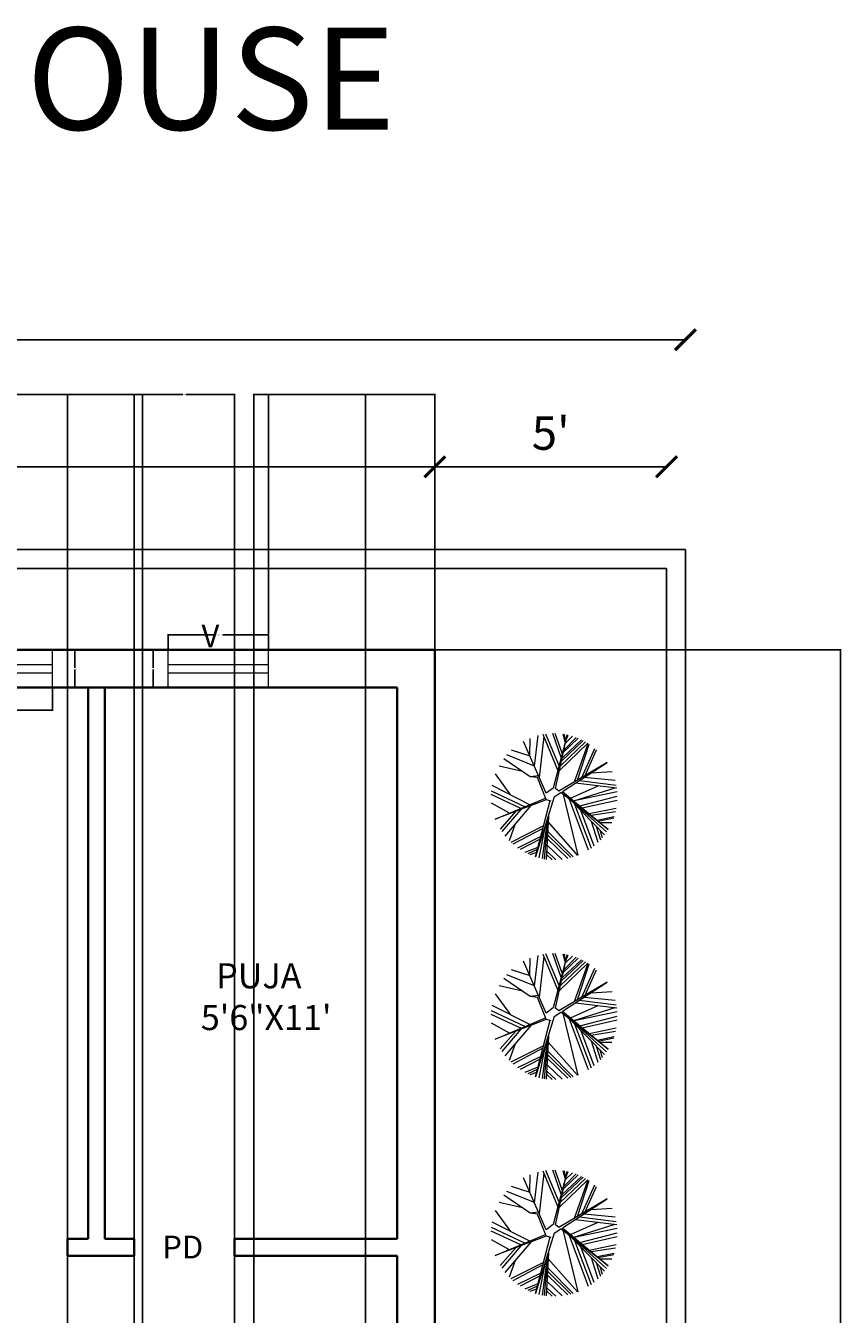
# Model space of a CAD drawing. Units: inches. Extents: x 503 to 1084, y -605 to 132.
# Tile 14 of 14: x 888 to 1084, y -177 to 132. Entities that reach past the tile are written whole.
import ezdxf

# ---------------------------------------------------------------- set-up
doc = ezdxf.new("R2010")
doc.units = ezdxf.units.IN
doc.header["$MEASUREMENT"] = 0
for name, color, linetype, lineweight in [('A-ANNO-DIMS', 7, 'Continuous', 18), ('A-ANNO-TEXT', 7, 'Continuous', 18), ('A-AREA-IDEN', 8, 'Continuous', 18), ('C-PROP', 1, 'Continuous', 25), ('wall', 1, 'Continuous', 35), ('wind', 5, 'Continuous', 18)]:
    doc.layers.add(name, color=color, linetype=linetype, lineweight=lineweight)
doc.layers.add('GRASS', color=90, linetype='Continuous', lineweight=13, transparency=0.7)
doc.styles.get("Standard").update_dxf_attribs({"font": 'arial.ttf'})
doc.dimstyles.get("Standard").update_dxf_attribs({"dimtxt": 0.18, "dimasz": 0.18, "dimexe": 0.18, "dimexo": 0.0625, "dimgap": 0.09, "dimtad": 0, "dimtih": 1, "dimtoh": 1, "dimdec": 1, "dimzin": 0, "dimdsep": 46, "dimlunit": 4, "dimtxsty": 'Standard', "dimcen": 0.09, "dimadec": 0, "dimazin": 0, "dimtfac": 1, "dimtdec": 1, "dimtofl": 0, "dimtmove": 0, "dimatfit": 3, "dimfxl": 1, "dimtolj": 1, "dimtzin": 0, "dimarcsym": 0})

# ---------------------------------------------------------------- blocks, each defined once
blk = doc.blocks.new('A$C4FA53466')
at = {"color": 0}
for p, q in [((0.717, 0.864), (0.422, 1.538)), ((0.501, 1.356), (0.505, 1.578)), ((0.563, 1.216), (0.612, 1.614)), ((0.627, 1.07), (0.687, 1.601)), ((0.867, 1.166), (0.675, 1.628)), ((0.882, 1.223), (0.709, 1.633)), ((0.91, 1.328), (0.802, 1.64)), ((0.988, 1.623), (0.804, 0.931)), ((0.925, 1.384), (0.834, 1.64)), ((0.836, 0.927), (0.988, 1.623)), ((0.887, 1.159), (1.256, 1.515)), ((0.901, 1.223), (1.228, 1.532)), ((0.914, 1.283), (1.197, 1.549)), ((0.922, 1.323), (1.176, 1.559)), ((0.964, 1.534), (0.938, 1.632)), ((0.938, 1.393), (1.132, 1.579)), ((0.945, 1.425), (1.104, 1.59)), ((0.967, 1.545), (0.952, 1.63)), ((0.965, 1.517), (1.059, 1.605)), ((0.974, 1.559), (1.002, 1.62)), ((1.085, 1.015), (1.262, 1.512)), ((0.562, 1.217), (0.205, 1.363)), ((0.505, 1.347), (0.266, 1.426)), ((1.121, 1.036), (1.274, 1.503)), ((1.18, 1.071), (1.349, 1.447)), ((1.222, 1.096), (1.37, 1.428)), ((0.406, 1.148), (0.102, 1.217)), ((0.506, 1.079), (0.165, 1.314)), ((1.509, 1.265), (0.879, 0.894)), ((0.926, 0.889), (1.509, 1.265)), ((0.255, 0.841), (0.055, 1.116)), ((0.614, 1.092), (0.506, 1.079)), ((0.604, 1.069), (0.506, 1.079)), ((0.715, 0.784), (0.604, 1.069)), ((1.148, 1.032), (1.626, 0.972)), ((1.211, 1.073), (1.612, 1.034)), ((1.3, 1.13), (1.573, 1.147)), ((0.384, 0.667), (0, 0.848)), ((0.436, 0.689), (0.003, 0.892)), ((0.501, 0.716), (0.012, 0.965)), ((0.804, 0.931), (0.717, 0.864)), ((0.82, 0.82), (0.904, 0.875)), ((0.879, 0.894), (0.836, 0.927)), ((1.521, 0.394), (0.904, 0.875)), ((0.926, 0.889), (1.521, 0.394)), ((0.938, 0.848), (1.126, 0.059)), ((1.03, 0.802), (1.392, 0.963)), ((1.073, 0.767), (1.614, 0.936)), ((1.081, 0.769), (1.638, 0.886)), ((1.097, 0.999), (1.632, 0.934)), ((0.237, 0.605), (0.004, 0.735)), ((0.053, 0.528), (0.708, 0.803)), ((0.716, 0.781), (0.053, 0.528)), ((0.516, 0.704), (0.179, 0.309)), ((0.82, 0.82), (0.575, 0.037)), ((0.575, 0.037), (0.769, 0.772)), ((0.715, 0.784), (0.775, 0.767)), ((1.016, 0.788), (1.263, 0.13)), ((1.04, 0.769), (1.475, 0.326)), ((1.06, 0.754), (1.5, 0.362)), ((1.083, 0.725), (1.298, 0.153)), ((1.153, 0.701), (1.64, 0.826)), ((1.185, 0.674), (1.639, 0.776)), ((1.273, 0.601), (1.627, 0.672)), ((0.321, 0.63), (0.115, 0.4)), ((0.387, 0.655), (0.137, 0.366)), ((0.732, 0.539), (0.664, 0.015)), ((0.737, 0.554), (0.691, 0.01)), ((0.744, 0.569), (0.717, 0.006)), ((1.161, 0.646), (1.335, 0.182)), ((1.298, 0.58), (1.618, 0.629)), ((1.301, 0.503), (1.386, 0.227)), ((1.376, 0.515), (1.599, 0.562)), ((1.392, 0.502), (1.593, 0.545)), ((0.313, 0.466), (0.232, 0.248)), ((0.682, 0.44), (0.255, 0.225)), ((0.673, 0.407), (0.281, 0.201)), ((0.701, 0.44), (0.621, 0.024)), ((0.735, 0.369), (1.067, 0.038)), ((0.74, 0.488), (1.121, 0.057)), ((1.365, 0.438), (1.42, 0.26)), ((1.412, 0.486), (1.569, 0.486)), ((1.413, 0.39), (1.444, 0.288)), ((0.645, 0.301), (0.342, 0.153)), ((0.636, 0.267), (0.375, 0.133)), ((0.726, 0.192), (0.924, 0.006)), ((0.73, 0.277), (0.998, 0.019)), ((0.733, 0.326), (1.037, 0.029)), ((0.608, 0.161), (0.439, 0.093)), ((0.6, 0.133), (0.475, 0.076)), ((0.59, 0.094), (0.501, 0.064)), ((0.72, 0.07), (0.793, 0)), ((0.722, 0.111), (0.842, 0))]:
    blk.add_line(p, q, dxfattribs=at)
blk = doc.blocks.new('_ArchTick')
at = {"color": 0, "linetype": 'ByBlock', "const_width": 0.15}
blk.add_lwpolyline([(-0.5, -0.5), (0.5, 0.5)], dxfattribs=at)
blk = doc.blocks.new('*D5')
at = {"layer": 'A-ANNO-DIMS', "color": 0, "lineweight": -3, "transparency": 16777216}
blk.add_line((590.09, 56.42), (1046.09, 56.42), dxfattribs=at)
at = {"layer": 'Defpoints', "color": 0, "transparency": 16777216}
for p in [(1046.09, 56.42), (590.09, 6.18), (1046.09, 6.18)]:
    blk.add_point(p, dxfattribs=at)
at = {"layer": 'A-ANNO-DIMS', "color": 0, "lineweight": -3, "transparency": 16777216, "xscale": 5, "yscale": 5, "zscale": 5, "rotation": 180}
blk.add_blockref('_ArchTick', (590.09, 56.42), dxfattribs=at)
at = {"layer": 'A-ANNO-DIMS', "color": 0, "lineweight": -3, "transparency": 16777216, "xscale": 5, "yscale": 5, "zscale": 5}
blk.add_blockref('_ArchTick', (1046.09, 56.42), dxfattribs=at)
at = {"layer": 'A-ANNO-DIMS', "color": 0, "transparency": 16777216, "insert": (818.09, 64.51), "char_height": 8, "attachment_point": 5}
blk.add_mtext("\\A1;38'", dxfattribs=at)
blk = doc.blocks.new('*D7')
at = {"layer": 'A-ANNO-DIMS', "color": 0, "lineweight": -3, "transparency": 16777216}
blk.add_line((650.09, 26.02), (986.09, 26.02), dxfattribs=at)
at = {"layer": 'Defpoints', "color": 0, "transparency": 16777216}
for p in [(986.09, 26.02), (650.09, -17.82), (986.09, -17.82)]:
    blk.add_point(p, dxfattribs=at)
at = {"layer": 'A-ANNO-DIMS', "color": 0, "lineweight": -3, "transparency": 16777216, "xscale": 5, "yscale": 5, "zscale": 5, "rotation": 180}
blk.add_blockref('_ArchTick', (650.09, 26.02), dxfattribs=at)
at = {"layer": 'A-ANNO-DIMS', "color": 0, "lineweight": -3, "transparency": 16777216, "xscale": 5, "yscale": 5, "zscale": 5}
blk.add_blockref('_ArchTick', (986.09, 26.02), dxfattribs=at)
at = {"layer": 'A-ANNO-DIMS', "color": 0, "transparency": 16777216, "insert": (818.09, 34.1), "char_height": 8, "attachment_point": 5}
blk.add_mtext("\\A1;28'", dxfattribs=at)
blk = doc.blocks.new('*D8')
at = {"layer": 'A-ANNO-DIMS', "color": 0, "lineweight": -3, "transparency": 16777216}
blk.add_line((986.09, 26.02), (1041.59, 26.02), dxfattribs=at)
at = {"layer": 'Defpoints', "color": 0, "transparency": 16777216}
for p in [(1041.59, 26.02), (986.09, -17.82), (1041.59, -17.14)]:
    blk.add_point(p, dxfattribs=at)
at = {"layer": 'A-ANNO-DIMS', "color": 0, "lineweight": -3, "transparency": 16777216, "xscale": 5, "yscale": 5, "zscale": 5, "rotation": 180}
blk.add_blockref('_ArchTick', (986.09, 26.02), dxfattribs=at)
at = {"layer": 'A-ANNO-DIMS', "color": 0, "lineweight": -3, "transparency": 16777216, "xscale": 5, "yscale": 5, "zscale": 5}
blk.add_blockref('_ArchTick', (1041.59, 26.02), dxfattribs=at)
at = {"layer": 'A-ANNO-DIMS', "color": 0, "transparency": 16777216, "insert": (1013.84, 34.09), "char_height": 8, "attachment_point": 5}
blk.add_mtext("\\A1;5'", dxfattribs=at)
blk = doc.blocks.new('WIN-36IN')
for p, q in [((0, 0), (0, 9)), ((36, 0), (36, 9)), ((0, 5.5), (36, 5.5)), ((0, 3.5), (36, 3.5))]:
    blk.add_line(p, q)
blk = doc.blocks.new('VENT-24IN')
for p, q in [((0, 9), (0, 0)), ((24, 9), (24, 0)), ((24, 5.5), (0, 5.5)), ((24, 3.5), (0, 3.5))]:
    blk.add_line(p, q)
blk = doc.blocks.new('*D22')
at = {"layer": 'A-ANNO-DIMS', "color": 0, "lineweight": -2, "transparency": 16777216}
for p, q in [((858.5, -26.88), (858.5, -32.4)), ((894.5, -26.88), (894.5, -32.4)), ((858.68, -32.22), (875.12, -32.22)), ((894.32, -32.22), (877.88, -32.22))]:
    blk.add_line(p, q, dxfattribs=at)
at = {"layer": 'A-ANNO-DIMS', "color": 0, "transparency": 16777216}
for points in [[(858.68, -32.19), (858.68, -32.25), (858.5, -32.22)], [(894.32, -32.19), (894.32, -32.25), (894.5, -32.22)]]:
    blk.add_solid(points, dxfattribs=at)
at = {"layer": 'Defpoints', "color": 0, "transparency": 16777216}
for p in [(858.5, -26.82), (894.5, -26.82), (894.5, -32.22)]:
    blk.add_point(p, dxfattribs=at)
at = {"layer": 'A-ANNO-DIMS', "color": 0, "transparency": 16777216, "insert": (876.5, -32.22), "char_height": 0.18, "attachment_point": 5}
blk.add_mtext('\\A1;WINDOW W 3\'-0" TYP.', dxfattribs=at)
blk = doc.blocks.new('*D23')
at = {"layer": 'A-ANNO-DIMS', "color": 0, "lineweight": -2, "transparency": 16777216}
for p, q in [((894.56, -17.82), (900.08, -17.82)), ((899.9, -18), (899.9, -22.13)), ((899.9, -26.64), (899.9, -22.5)), ((894.56, -26.82), (900.08, -26.82))]:
    blk.add_line(p, q, dxfattribs=at)
at = {"layer": 'A-ANNO-DIMS', "color": 0, "transparency": 16777216}
for points in [[(899.87, -18), (899.93, -18), (899.9, -17.82)], [(899.87, -26.64), (899.93, -26.64), (899.9, -26.82)]]:
    blk.add_solid(points, dxfattribs=at)
at = {"layer": 'Defpoints', "color": 0, "transparency": 16777216}
for p in [(894.5, -17.82), (899.9, -17.82), (894.5, -26.82)]:
    blk.add_point(p, dxfattribs=at)
at = {"layer": 'A-ANNO-DIMS', "color": 0, "transparency": 16777216, "insert": (899.9, -22.32), "char_height": 0.18, "attachment_point": 5}
blk.add_mtext('\\A1;0\'-9" TYP.', dxfattribs=at)
blk = doc.blocks.new('*D24')
at = {"layer": 'A-ANNO-DIMS', "color": 0, "lineweight": -2, "transparency": 16777216}
for p, q in [((922.22, -17.75), (922.22, -14.04)), ((922.4, -14.22), (933.09, -14.22)), ((946.04, -14.22), (935.35, -14.22)), ((946.22, -17.75), (946.22, -14.04))]:
    blk.add_line(p, q, dxfattribs=at)
at = {"layer": 'A-ANNO-DIMS', "color": 0, "transparency": 16777216}
for points in [[(922.4, -14.19), (922.4, -14.25), (922.22, -14.22)], [(946.04, -14.19), (946.04, -14.25), (946.22, -14.22)]]:
    blk.add_solid(points, dxfattribs=at)
at = {"layer": 'Defpoints', "color": 0, "transparency": 16777216}
for p in [(922.22, -14.22), (922.22, -17.82), (946.22, -17.82)]:
    blk.add_point(p, dxfattribs=at)
at = {"layer": 'A-ANNO-DIMS', "color": 0, "transparency": 16777216, "insert": (934.22, -14.22), "char_height": 0.18, "attachment_point": 5}
blk.add_mtext('\\A1;VENT V 2\'-0" TYP.', dxfattribs=at)
blk = doc.blocks.new('*D25')
at = {"layer": 'A-ANNO-DIMS', "color": 0, "lineweight": -2, "transparency": 16777216}
for p, q in [((922.16, -17.82), (918.44, -17.82)), ((918.62, -18), (918.62, -22.13)), ((918.62, -26.64), (918.62, -22.5)), ((922.16, -26.82), (918.44, -26.82))]:
    blk.add_line(p, q, dxfattribs=at)
at = {"layer": 'A-ANNO-DIMS', "color": 0, "transparency": 16777216}
for points in [[(918.59, -18), (918.65, -18), (918.62, -17.82)], [(918.59, -26.64), (918.65, -26.64), (918.62, -26.82)]]:
    blk.add_solid(points, dxfattribs=at)
at = {"layer": 'Defpoints', "color": 0, "transparency": 16777216}
for p in [(922.22, -17.82), (918.62, -26.82), (922.22, -26.82)]:
    blk.add_point(p, dxfattribs=at)
at = {"layer": 'A-ANNO-DIMS', "color": 0, "transparency": 16777216, "insert": (918.62, -22.32), "char_height": 0.18, "attachment_point": 5}
blk.add_mtext('\\A1;0\'-9" TYP.', dxfattribs=at)
blk = doc.blocks.new('*D42')
at = {"layer": 'A-ANNO-DIMS', "color": 0, "lineweight": -2, "transparency": 16777216}
for p, q in [((986.15, -17.82), (1083.42, -17.82)), ((1083.24, -18), (1083.24, -190.63)), ((1083.24, -363.64), (1083.24, -191)), ((986.15, -363.82), (1083.42, -363.82))]:
    blk.add_line(p, q, dxfattribs=at)
at = {"layer": 'A-ANNO-DIMS', "color": 0, "transparency": 16777216}
for points in [[(1083.21, -18), (1083.27, -18), (1083.24, -17.82)], [(1083.21, -363.64), (1083.27, -363.64), (1083.24, -363.82)]]:
    blk.add_solid(points, dxfattribs=at)
at = {"layer": 'Defpoints', "color": 0, "transparency": 16777216}
for p in [(986.09, -17.82), (1083.24, -17.82), (986.09, -363.82)]:
    blk.add_point(p, dxfattribs=at)
at = {"layer": 'A-ANNO-DIMS', "color": 0, "transparency": 16777216, "insert": (1083.24, -190.82), "char_height": 0.18, "attachment_point": 5}
blk.add_mtext('\\A1;28\'-10"', dxfattribs=at)
blk = doc.blocks.new('*D45')
at = {"layer": 'A-ANNO-DIMS', "color": 0, "lineweight": -2, "transparency": 16777216}
for p, q in [((844.09, -354.75), (844.09, 43.51)), ((844.27, 43.33), (879.76, 43.33)), ((915.91, 43.33), (880.42, 43.33)), ((916.09, -354.75), (916.09, 43.51))]:
    blk.add_line(p, q, dxfattribs=at)
at = {"layer": 'A-ANNO-DIMS', "color": 0, "transparency": 16777216}
for points in [[(844.27, 43.36), (844.27, 43.3), (844.09, 43.33)], [(915.91, 43.36), (915.91, 43.3), (916.09, 43.33)]]:
    blk.add_solid(points, dxfattribs=at)
at = {"layer": 'Defpoints', "color": 0, "transparency": 16777216}
for p in [(916.09, 43.33), (844.09, -354.82), (916.09, -354.82)]:
    blk.add_point(p, dxfattribs=at)
at = {"layer": 'A-ANNO-DIMS', "color": 0, "transparency": 16777216, "insert": (880.09, 43.33), "char_height": 0.18, "attachment_point": 5}
blk.add_mtext('\\A1;6\'-0"', dxfattribs=at)
blk = doc.blocks.new('*D51')
at = {"layer": 'A-ANNO-DIMS', "color": 0, "lineweight": -2, "transparency": 16777216}
for p, q in [((946.22, -17.75), (946.22, 43.51)), ((946.4, 43.33), (965.83, 43.33)), ((985.91, 43.33), (966.48, 43.33)), ((986.09, -17.75), (986.09, 43.51))]:
    blk.add_line(p, q, dxfattribs=at)
at = {"layer": 'A-ANNO-DIMS', "color": 0, "transparency": 16777216}
for points in [[(946.4, 43.36), (946.4, 43.3), (946.22, 43.33)], [(985.91, 43.36), (985.91, 43.3), (986.09, 43.33)]]:
    blk.add_solid(points, dxfattribs=at)
at = {"layer": 'Defpoints', "color": 0, "transparency": 16777216}
for p in [(986.09, 43.33), (946.22, -17.82), (986.09, -17.82)]:
    blk.add_point(p, dxfattribs=at)
at = {"layer": 'A-ANNO-DIMS', "color": 0, "transparency": 16777216, "insert": (966.15, 43.33), "char_height": 0.18, "attachment_point": 5}
blk.add_mtext('\\A1;3\'-4"', dxfattribs=at)
blk = doc.blocks.new('*D57')
at = {"layer": 'A-ANNO-DIMS', "color": 0, "lineweight": -2, "transparency": 16777216}
for p, q in [((868.09, -162.75), (868.09, 43.51)), ((868.27, 43.33), (882.76, 43.33)), ((897.91, 43.33), (883.42, 43.33)), ((898.09, -162.75), (898.09, 43.51))]:
    blk.add_line(p, q, dxfattribs=at)
at = {"layer": 'A-ANNO-DIMS', "color": 0, "transparency": 16777216}
for points in [[(868.27, 43.36), (868.27, 43.3), (868.09, 43.33)], [(897.91, 43.36), (897.91, 43.3), (898.09, 43.33)]]:
    blk.add_solid(points, dxfattribs=at)
at = {"layer": 'Defpoints', "color": 0, "transparency": 16777216}
for p in [(898.09, 43.33), (868.09, -162.82), (898.09, -162.82)]:
    blk.add_point(p, dxfattribs=at)
at = {"layer": 'A-ANNO-DIMS', "color": 0, "transparency": 16777216, "insert": (883.09, 43.33), "char_height": 0.18, "attachment_point": 5}
blk.add_mtext('\\A1;2\'-6"', dxfattribs=at)
blk = doc.blocks.new('*D58')
at = {"layer": 'A-ANNO-DIMS', "color": 0, "lineweight": -2, "transparency": 16777216}
for p, q in [((914.09, -162.75), (914.09, 43.51)), ((914.27, 43.33), (925.76, 43.33)), ((937.91, 43.33), (926.42, 43.33)), ((938.09, -162.75), (938.09, 43.51))]:
    blk.add_line(p, q, dxfattribs=at)
at = {"layer": 'A-ANNO-DIMS', "color": 0, "transparency": 16777216}
for points in [[(914.27, 43.36), (914.27, 43.3), (914.09, 43.33)], [(937.91, 43.36), (937.91, 43.3), (938.09, 43.33)]]:
    blk.add_solid(points, dxfattribs=at)
at = {"layer": 'Defpoints', "color": 0, "transparency": 16777216}
for p in [(938.09, 43.33), (914.09, -162.82), (938.09, -162.82)]:
    blk.add_point(p, dxfattribs=at)
at = {"layer": 'A-ANNO-DIMS', "color": 0, "transparency": 16777216, "insert": (926.09, 43.33), "char_height": 0.18, "attachment_point": 5}
blk.add_mtext('\\A1;2\'-0"', dxfattribs=at)
blk = doc.blocks.new('*D64')
at = {"layer": 'A-ANNO-DIMS', "color": 0, "lineweight": -2, "transparency": 16777216}
for p, q in [((938.09, -162.88), (938.09, -583.15)), ((977.09, -162.88), (977.09, -583.15)), ((938.27, -582.97), (957.26, -582.97)), ((976.91, -582.97), (957.92, -582.97))]:
    blk.add_line(p, q, dxfattribs=at)
at = {"layer": 'A-ANNO-DIMS', "color": 0, "transparency": 16777216}
for points in [[(938.27, -582.94), (938.27, -583), (938.09, -582.97)], [(976.91, -582.94), (976.91, -583), (977.09, -582.97)]]:
    blk.add_solid(points, dxfattribs=at)
at = {"layer": 'Defpoints', "color": 0, "transparency": 16777216}
for p in [(938.09, -162.82), (977.09, -162.82), (977.09, -582.97)]:
    blk.add_point(p, dxfattribs=at)
at = {"layer": 'A-ANNO-DIMS', "color": 0, "transparency": 16777216, "insert": (957.59, -582.97), "char_height": 0.18, "attachment_point": 5}
blk.add_mtext('\\A1;3\'-3"', dxfattribs=at)
blk = doc.blocks.new('*D65')
at = {"layer": 'A-ANNO-DIMS', "color": 0, "lineweight": -2, "transparency": 16777216}
for p, q in [((898.09, -162.88), (898.09, -583.15)), ((914.09, -162.88), (914.09, -583.15)), ((898.27, -582.97), (905.77, -582.97)), ((913.91, -582.97), (906.41, -582.97))]:
    blk.add_line(p, q, dxfattribs=at)
at = {"layer": 'A-ANNO-DIMS', "color": 0, "transparency": 16777216}
for points in [[(898.27, -582.94), (898.27, -583), (898.09, -582.97)], [(913.91, -582.94), (913.91, -583), (914.09, -582.97)]]:
    blk.add_solid(points, dxfattribs=at)
at = {"layer": 'Defpoints', "color": 0, "transparency": 16777216}
for p in [(898.09, -162.82), (914.09, -162.82), (914.09, -582.97)]:
    blk.add_point(p, dxfattribs=at)
at = {"layer": 'A-ANNO-DIMS', "color": 0, "transparency": 16777216, "insert": (906.09, -582.97), "char_height": 0.18, "attachment_point": 5}
blk.add_mtext('\\A1;1\'-4"', dxfattribs=at)
blk = doc.blocks.new('*D71')
at = {"layer": 'A-ANNO-DIMS', "color": 0, "lineweight": -2, "transparency": 16777216}
for p, q in [((942.75, -236.15), (942.75, 43.51)), ((942.93, 43.33), (955.57, 43.33)), ((969.29, 43.33), (956.65, 43.33)), ((969.47, -235.11), (969.47, 43.51))]:
    blk.add_line(p, q, dxfattribs=at)
at = {"layer": 'A-ANNO-DIMS', "color": 0, "transparency": 16777216}
for points in [[(942.93, 43.36), (942.93, 43.3), (942.75, 43.33)], [(969.29, 43.36), (969.29, 43.3), (969.47, 43.33)]]:
    blk.add_solid(points, dxfattribs=at)
at = {"layer": 'Defpoints', "color": 0, "transparency": 16777216}
for p in [(969.47, 43.33), (942.75, -236.21), (969.47, -235.17)]:
    blk.add_point(p, dxfattribs=at)
at = {"layer": 'A-ANNO-DIMS', "color": 0, "transparency": 16777216, "insert": (956.11, 43.33), "char_height": 0.18, "attachment_point": 5}
blk.add_mtext('\\A1;2\'-2 1/2"', dxfattribs=at)

msp = doc.modelspace()

# ---------------------------------------------------------------- linework, layer by layer
at = {"layer": 'C-PROP'}
for p, q in [((590.09, 6.18), (1046.09, 6.18)), ((1046.09, 6.18), (1046.09, -545.82)), ((1041.59, 1.68), (594.59, 1.68)), ((1041.59, -541.32), (1041.59, 1.68))]:
    msp.add_line(p, q, dxfattribs=at)
at = {"layer": 'wall'}
for p, q in [((650.09, -17.82), (986.09, -17.82)), ((986.09, -17.82), (986.09, -363.82)), ((659.09, -26.82), (977.09, -26.82)), ((903.09, -26.82), (903.09, -158.82)), ((907.09, -26.82), (907.09, -158.82)), ((977.09, -26.82), (977.09, -158.82)), ((898.09, -158.82), (898.09, -162.82)), ((898.09, -158.82), (903.09, -158.82)), ((907.09, -158.82), (914.09, -158.82)), ((914.09, -158.82), (914.09, -162.82)), ((938.09, -158.82), (938.09, -162.82)), ((938.09, -158.82), (977.09, -158.82)), ((898.09, -162.82), (914.09, -162.82)), ((938.09, -162.82), (977.09, -162.82)), ((977.09, -162.82), (977.09, -354.82))]:
    msp.add_line(p, q, dxfattribs=at)

# ---------------------------------------------------------------- block references
at = {"layer": 'GRASS', "xscale": 18.41745235960633, "yscale": 18.41745235960633, "zscale": 18.41745235960633}
for p in [(999.58, -68.06), (999.58, -120.68), (999.58, -172.54)]:
    msp.add_blockref('A$C4FA53466', p, dxfattribs=at)
at = {"layer": 'wind'}
msp.add_blockref('WIN-36IN', (858.51, -26.82), dxfattribs=at)
at = {"layer": 'wind', "rotation": 180}
msp.add_blockref('VENT-24IN', (946.22, -17.81), dxfattribs=at)

# ---------------------------------------------------------------- texts
at = {"layer": 'A-ANNO-TEXT'}
for s, height, p in [('V', 5.44, (930.21, -17.2)), ('PD', 5.444, (920.81, -163.48))]:
    msp.add_text(s, height=height, dxfattribs=at).set_placement(p)
at = {"layer": 'A-ANNO-TEXT', "insert": (619.28, 131.14), "char_height": 24.4528, "attachment_point": 1}
msp.add_mtext_dynamic_manual_height_columns('SOUTH FACING HOUSE', width=395.3147, gutter_width=4.08, heights=[0], dxfattribs=at)
at = {"layer": 'A-AREA-IDEN', "insert": (922.71, -92.82), "char_height": 6, "attachment_point": 1}
msp.add_mtext_dynamic_manual_height_columns('      PUJA\\P    5\'6"X11\'', width=43.0051, gutter_width=1, heights=[0], dxfattribs=at)

# ---------------------------------------------------------------- dimensions: what is measured, and where the dimension line sits
at = {"layer": 'A-ANNO-DIMS'}
for base, p1, p2, override, picture, middle in [((1046.09, 56.42), (590.09, 6.18), (1046.09, 6.18), {"dimtxt": 8, "dimasz": 5, "dimgap": 4, "dimtad": 1, "dimblk1": 'ArchTick', "dimblk2": 'ArchTick', "dimsah": 1, "dimse1": 1, "dimse2": 1, "dimclrd": 0, "dimclre": 0, "dimclrt": 0, "dimlwd": -3}, '*D5', (818.09, 64.51)), ((916.09, 43.33), (844.09, -354.82), (916.09, -354.82), {"dimdec": 1, "dimlfac": 1, "dimrnd": 0, "dimzin": 1, "dimdsep": 46, "dimlunit": 4, "dimfrac": 2}, '*D45', (880.09, 43.33)), ((898.09, 43.33), (868.09, -162.82), (898.09, -162.82), {"dimdec": 1, "dimlfac": 1, "dimrnd": 0, "dimzin": 1, "dimdsep": 46, "dimlunit": 4, "dimfrac": 2}, '*D57', (883.09, 43.33)), ((938.09, 43.33), (914.09, -162.82), (938.09, -162.82), {"dimdec": 1, "dimlfac": 1, "dimrnd": 0, "dimzin": 1, "dimdsep": 46, "dimlunit": 4, "dimfrac": 2}, '*D58', (926.09, 43.33)), ((969.47, 43.33), (942.75, -236.21), (969.47, -235.17), {"dimdec": 1, "dimlfac": 1, "dimrnd": 0, "dimzin": 1, "dimdsep": 46, "dimlunit": 4, "dimfrac": 2}, '*D71', (956.11, 43.33)), ((986.09, 43.33), (946.22, -17.82), (986.09, -17.82), {"dimdec": 1, "dimlfac": 1, "dimrnd": 0, "dimzin": 1, "dimdsep": 46, "dimlunit": 4, "dimfrac": 2}, '*D51', (966.15, 43.33)), ((986.09, 26.02), (650.09, -17.82), (986.09, -17.82), {"dimtxt": 8, "dimasz": 5, "dimgap": 4, "dimtad": 1, "dimblk1": 'ArchTick', "dimblk2": 'ArchTick', "dimsah": 1, "dimse1": 1, "dimse2": 1, "dimclrd": 0, "dimclre": 0, "dimclrt": 0, "dimlwd": -3}, '*D7', (818.09, 34.1)), ((914.09, -582.97), (898.09, -162.82), (914.09, -162.82), {"dimdec": 1, "dimlfac": 1, "dimrnd": 0, "dimzin": 1, "dimdsep": 46, "dimlunit": 4, "dimfrac": 2}, '*D65', (906.09, -582.97)), ((977.09, -582.97), (938.09, -162.82), (977.09, -162.82), {"dimdec": 1, "dimlfac": 1, "dimrnd": 0, "dimzin": 1, "dimdsep": 46, "dimlunit": 4, "dimfrac": 2}, '*D64', (957.59, -582.97))]:
    dim = msp.add_linear_dim(base=base, p1=p1, p2=p2, dimstyle='Standard', override=override, dxfattribs=at)
    dim.commit()
    dim.dimension.update_dxf_attribs({"geometry": picture, "text_midpoint": middle})
for base, p1, p2, text, override, picture, middle in [((1041.59, 26.02), (986.09, -17.82), (1041.59, -17.14), "5'", {"dimtxt": 8, "dimasz": 5, "dimgap": 4, "dimtad": 1, "dimblk1": 'ArchTick', "dimblk2": 'ArchTick', "dimsah": 1, "dimse1": 1, "dimse2": 1, "dimclrd": 0, "dimclre": 0, "dimclrt": 0, "dimlwd": -3}, '*D8', (1013.84, 34.09)), ((894.5, -32.22), (858.5, -26.82), (894.5, -26.82), 'WINDOW W <> TYP.', {"dimdec": 1, "dimlfac": 1, "dimrnd": 0, "dimzin": 1, "dimdsep": 46, "dimlunit": 4, "dimfrac": 2}, '*D22', (876.5, -32.22))]:
    dim = msp.add_linear_dim(base=base, p1=p1, p2=p2, text=text, dimstyle='Standard', override=override, dxfattribs=at)
    dim.commit()
    dim.dimension.update_dxf_attribs({"geometry": picture, "text_midpoint": middle})
for base, p1, p2, angle, text, picture, middle in [((922.22, -14.22), (946.22, -17.82), (922.22, -17.82), 180, 'VENT V <> TYP.', '*D24', (934.22, -14.22)), ((899.9, -17.82), (894.5, -26.82), (894.5, -17.82), 90, '<> TYP.', '*D23', (899.9, -22.32)), ((918.62, -26.82), (922.22, -17.82), (922.22, -26.82), 270, '<> TYP.', '*D25', (918.62, -22.32))]:
    dim = msp.add_linear_dim(base=base, p1=p1, p2=p2, angle=angle, text=text, dimstyle='Standard', override={"dimdec": 1, "dimlfac": 1, "dimrnd": 0, "dimzin": 1, "dimdsep": 46, "dimlunit": 4, "dimfrac": 2}, dxfattribs=at)
    dim.commit()
    dim.dimension.update_dxf_attribs({"geometry": picture, "text_midpoint": middle})
dim = msp.add_linear_dim(base=(1083.24, -17.82), p1=(986.09, -363.82), p2=(986.09, -17.82), angle=90, dimstyle='Standard', override={"dimdec": 1, "dimlfac": 1, "dimrnd": 0, "dimzin": 1, "dimdsep": 46, "dimlunit": 4, "dimfrac": 2}, dxfattribs=at)
dim.commit()
dim.dimension.update_dxf_attribs({"geometry": '*D42', "text_midpoint": (1083.24, -190.82)})

doc.saveas('drawing.dxf')
